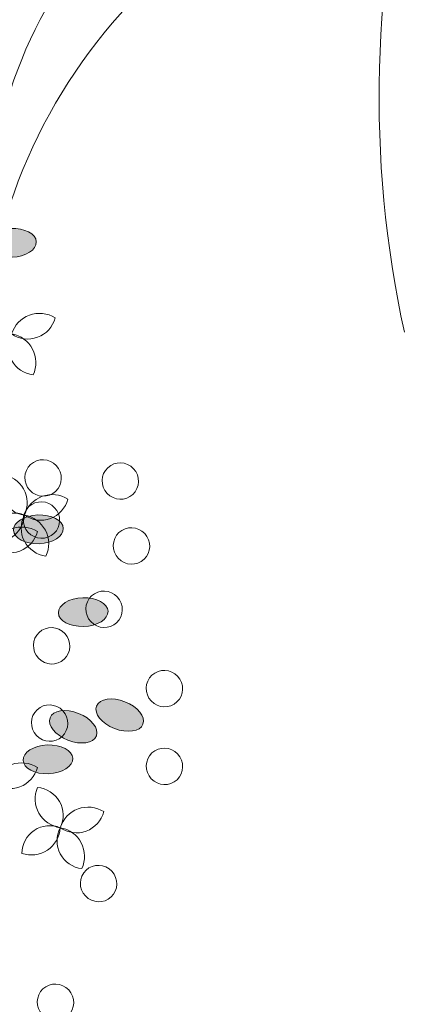
# Model space of a CAD drawing. Units: millimetres. Extents: x 595116 to 630915, y 909473 to 920225.
# Tile 47 of 134: x 629519 to 629529, y 919255 to 919281. Entities that reach past the tile are written whole.
import ezdxf

# ---------------------------------------------------------------- set-up
doc = ezdxf.new("R2010")
doc.units = ezdxf.units.MM
doc.layers.add('Dimension', color=3, linetype='Continuous', lineweight=18)
doc.layers.add('L-PLNT', color=85, linetype='Continuous', lineweight=13)
doc.styles.get("Standard").update_dxf_attribs({"font": 'arial.ttf'})
doc.dimstyles.new('ISO-25', dxfattribs={"dimtxt": 9, "dimasz": 6, "dimexe": 1.25, "dimexo": 0.625, "dimtad": 1, "dimlunit": 4, "dimtxsty": 'Standard', "dimcen": 2.5, "dimadec": 0, "dimazin": 0, "dimtfac": 1, "dimtmove": 0, "dimatfit": 3, "dimfxl": 1, "dimarcsym": 0})

# ---------------------------------------------------------------- blocks, each defined once
blk = doc.blocks.new('tree')
for centre, radius, start, end in [((629598.153, 919288.998), 5.103, 105.3576, 208.8973), ((629601.247, 919287.941), 5.545, 101.0419, 191.8692), ((629614.329, 919289.554), 13.748, 164.5925, 192.323), ((629602.391, 919286.088), 6.769, 99.681, 184.5451)]:
    blk.add_arc(centre, radius, start, end)
blk = doc.blocks.new('A$C77972600')
h = blk.add_hatch(color=256)
edge = h.paths.add_edge_path()
edge.add_ellipse((3.0705, 5.8276), major_axis=(-0.1731, 0.0699), ratio=0.578492, start_angle=0, end_angle=360)
edge = h.paths.add_edge_path()
edge.add_ellipse((4.0989, 6.0027), major_axis=(-0.1319, 0.1321), ratio=0.578492, start_angle=0, end_angle=360)
edge = h.paths.add_edge_path()
edge.add_ellipse((4.5318, 6.7683), major_axis=(-0.1688, -0.0798), ratio=0.578492, start_angle=0, end_angle=360)
edge = h.paths.add_edge_path()
edge.add_ellipse((5.185, 6.8705), major_axis=(-0.1865, -0.0073), ratio=0.578492, start_angle=0, end_angle=360)
edge = h.paths.add_edge_path()
edge.add_ellipse((4.6885, 3.4464), major_axis=(-0.1865, -0.0073), ratio=0.578492, start_angle=0, end_angle=360)
edge = h.paths.add_edge_path()
edge.add_ellipse((4.5217, 4.2367), major_axis=(-0.1865, -0.0073), ratio=0.578492, start_angle=0, end_angle=360)
edge = h.paths.add_edge_path()
edge.add_ellipse((4.9166, 3.9946), major_axis=(-0.1731, 0.0699), ratio=0.578492, start_angle=0, end_angle=360)
edge = h.paths.add_edge_path()
edge.add_ellipse((3.6759, 4.9988), major_axis=(-0.1319, 0.1321), ratio=0.578492, start_angle=0, end_angle=360)
edge = h.paths.add_edge_path()
edge.add_ellipse((3.1035, 4.6784), major_axis=(-0.1319, 0.1321), ratio=0.578492, start_angle=0, end_angle=360)
edge = h.paths.add_edge_path()
edge.add_ellipse((3.8133, 4.5577), major_axis=(-0.1319, 0.1321), ratio=0.578492, start_angle=0, end_angle=360)
edge = h.paths.add_edge_path()
edge.add_ellipse((2.2042, 5.6327), major_axis=(-0.1865, -0.0073), ratio=0.578492, start_angle=0, end_angle=360)
edge = h.paths.add_edge_path()
edge.add_ellipse((2.9066, 5.6543), major_axis=(-0.1865, -0.0073), ratio=0.578492, start_angle=0, end_angle=360)
edge = h.paths.add_edge_path()
edge.add_ellipse((2.6215, 5.4344), major_axis=(-0.1865, -0.0073), ratio=0.578492, start_angle=0, end_angle=360)
edge = h.paths.add_edge_path()
edge.add_ellipse((2.1195, 4.0174), major_axis=(-0.1731, 0.0699), ratio=0.578492, start_angle=0, end_angle=360)
edge = h.paths.add_edge_path()
edge.add_ellipse((4.1491, 5.5914), major_axis=(-0.1688, -0.0798), ratio=0.578492, start_angle=0, end_angle=360)
edge = h.paths.add_edge_path()
edge.add_ellipse((1.9571, 3.173), major_axis=(-0.1865, -0.0073), ratio=0.578492, start_angle=0, end_angle=360)
edge = h.paths.add_edge_path()
edge.add_ellipse((1.589, 3.2907), major_axis=(-0.1688, -0.0798), ratio=0.578492, start_angle=0, end_angle=360)
edge = h.paths.add_edge_path()
edge.add_ellipse((1.045, 3.0811), major_axis=(-0.1865, -0.0073), ratio=0.578492, start_angle=0, end_angle=360)
edge = h.paths.add_edge_path()
edge.add_ellipse((1.2104, 3.7739), major_axis=(-0.1688, -0.0798), ratio=0.578492, start_angle=0, end_angle=360)
edge = h.paths.add_edge_path()
edge.add_ellipse((1.6721, 3.755), major_axis=(-0.1688, -0.0798), ratio=0.578492, start_angle=0, end_angle=360)
edge = h.paths.add_edge_path()
edge.add_ellipse((0.772, 4.473), major_axis=(-0.1731, 0.0699), ratio=0.578492, start_angle=0, end_angle=360)
edge = h.paths.add_edge_path()
edge.add_ellipse((0.8326, 5.2916), major_axis=(-0.1319, 0.1321), ratio=0.578492, start_angle=0, end_angle=360)
edge = h.paths.add_edge_path()
edge.add_ellipse((1.1875, 5.2313), major_axis=(-0.1319, 0.1321), ratio=0.578492, start_angle=0, end_angle=360)
edge = h.paths.add_edge_path()
edge.add_ellipse((5.3876, 4.7197), major_axis=(-0.1865, -0.0073), ratio=0.578492, start_angle=0, end_angle=360)
edge = h.paths.add_edge_path()
edge.add_ellipse((3.5552, 2.162), major_axis=(-0.1865, -0.0073), ratio=0.578492, start_angle=0, end_angle=360)
edge = h.paths.add_edge_path()
edge.add_ellipse((3.8402, 2.3819), major_axis=(-0.1865, -0.0073), ratio=0.578492, start_angle=0, end_angle=360)
edge = h.paths.add_edge_path()
edge.add_ellipse((4.692, 2.204), major_axis=(-0.1731, 0.0699), ratio=0.578492, start_angle=0, end_angle=360)
edge = h.paths.add_edge_path()
edge.add_ellipse((4.514, 2.9096), major_axis=(-0.1731, 0.0699), ratio=0.578492, start_angle=0, end_angle=360)
edge = h.paths.add_edge_path()
edge.add_ellipse((4.8133, 2.5575), major_axis=(-0.1731, 0.0699), ratio=0.578492, start_angle=0, end_angle=360)
edge = h.paths.add_edge_path()
edge.add_ellipse((3.7876, 2.8899), major_axis=(-0.1731, 0.0699), ratio=0.578492, start_angle=0, end_angle=360)
h = blk.add_hatch(color=256)
edge = h.paths.add_edge_path()
edge.add_ellipse((3.2403, 1.6985), major_axis=(-0.1668, -0.0838), ratio=0.578492, start_angle=0, end_angle=360, ccw=False)
edge = h.paths.add_edge_path()
edge.add_ellipse((4.2796, 1.6084), major_axis=(-0.1206, -0.1425), ratio=0.578492, start_angle=0, end_angle=360, ccw=False)
edge = h.paths.add_edge_path()
edge.add_ellipse((4.7739, 0.881), major_axis=(-0.1747, 0.0657), ratio=0.578492, start_angle=0, end_angle=360, ccw=False)
edge = h.paths.add_edge_path()
edge.add_ellipse((5.4333, 0.8328), major_axis=(-0.1865, -0.008), ratio=0.578492, start_angle=0, end_angle=360, ccw=False)
edge = h.paths.add_edge_path()
edge.add_ellipse((4.6573, 4.2045), major_axis=(-0.1865, -0.008), ratio=0.578492, start_angle=0, end_angle=360, ccw=False)
edge = h.paths.add_edge_path()
edge.add_ellipse((4.556, 3.4032), major_axis=(-0.1865, -0.008), ratio=0.578492, start_angle=0, end_angle=360, ccw=False)
edge = h.paths.add_edge_path()
edge.add_ellipse((4.9297, 3.677), major_axis=(-0.1668, -0.0838), ratio=0.578492, start_angle=0, end_angle=360, ccw=False)
edge = h.paths.add_edge_path()
edge.add_ellipse((3.7756, 2.5742), major_axis=(-0.1206, -0.1425), ratio=0.578492, start_angle=0, end_angle=360, ccw=False)
edge = h.paths.add_edge_path()
edge.add_ellipse((3.1788, 2.8466), major_axis=(-0.1206, -0.1425), ratio=0.578492, start_angle=0, end_angle=360, ccw=False)
edge = h.paths.add_edge_path()
edge.add_ellipse((3.8763, 3.0252), major_axis=(-0.1206, -0.1425), ratio=0.578492, start_angle=0, end_angle=360, ccw=False)
edge = h.paths.add_edge_path()
edge.add_ellipse((2.3609, 1.8217), major_axis=(-0.1865, -0.008), ratio=0.578492, start_angle=0, end_angle=360, ccw=False)
edge = h.paths.add_edge_path()
edge.add_ellipse((3.0627, 1.8578), major_axis=(-0.1865, -0.008), ratio=0.578492, start_angle=0, end_angle=360, ccw=False)
edge = h.paths.add_edge_path()
edge.add_ellipse((2.7605, 2.0535), major_axis=(-0.1865, -0.008), ratio=0.578492, start_angle=0, end_angle=360, ccw=False)
edge = h.paths.add_edge_path()
edge.add_ellipse((2.1439, 3.4246), major_axis=(-0.1668, -0.0838), ratio=0.578492, start_angle=0, end_angle=360, ccw=False)
edge = h.paths.add_edge_path()
edge.add_ellipse((4.2959, 2.0225), major_axis=(-0.1747, 0.0657), ratio=0.578492, start_angle=0, end_angle=360, ccw=False)
edge = h.paths.add_edge_path()
edge.add_ellipse((1.9127, 4.2528), major_axis=(-0.1865, -0.008), ratio=0.578492, start_angle=0, end_angle=360, ccw=False)
edge = h.paths.add_edge_path()
edge.add_ellipse((1.5555, 4.1052), major_axis=(-0.1747, 0.0657), ratio=0.578492, start_angle=0, end_angle=360, ccw=False)
edge = h.paths.add_edge_path()
edge.add_ellipse((0.9962, 4.2695), major_axis=(-0.1865, -0.008), ratio=0.578492, start_angle=0, end_angle=360, ccw=False)
edge = h.paths.add_edge_path()
edge.add_ellipse((1.2179, 3.5926), major_axis=(-0.1747, 0.0657), ratio=0.578492, start_angle=0, end_angle=360, ccw=False)
edge = h.paths.add_edge_path()
edge.add_ellipse((1.6764, 3.6493), major_axis=(-0.1747, 0.0657), ratio=0.578492, start_angle=0, end_angle=360, ccw=False)
edge = h.paths.add_edge_path()
edge.add_ellipse((0.8384, 2.8599), major_axis=(-0.1668, -0.0838), ratio=0.578492, start_angle=0, end_angle=360, ccw=False)
edge = h.paths.add_edge_path()
edge.add_ellipse((0.9659, 2.049), major_axis=(-0.1206, -0.1425), ratio=0.578492, start_angle=0, end_angle=360, ccw=False)
edge = h.paths.add_edge_path()
edge.add_ellipse((1.3147, 2.1383), major_axis=(-0.1206, -0.1425), ratio=0.578492, start_angle=0, end_angle=360, ccw=False)
edge = h.paths.add_edge_path()
edge.add_ellipse((5.4586, 2.9929), major_axis=(-0.1865, -0.008), ratio=0.578492, start_angle=0, end_angle=360, ccw=False)
edge = h.paths.add_edge_path()
edge.add_ellipse((3.4224, 5.3915), major_axis=(-0.1865, -0.008), ratio=0.578492, start_angle=0, end_angle=360, ccw=False)
edge = h.paths.add_edge_path()
edge.add_ellipse((3.7245, 5.1958), major_axis=(-0.1865, -0.008), ratio=0.578492, start_angle=0, end_angle=360, ccw=False)
edge = h.paths.add_edge_path()
edge.add_ellipse((4.5588, 5.4431), major_axis=(-0.1668, -0.0838), ratio=0.578492, start_angle=0, end_angle=360, ccw=False)
edge = h.paths.add_edge_path()
edge.add_ellipse((4.4393, 4.7252), major_axis=(-0.1668, -0.0838), ratio=0.578492, start_angle=0, end_angle=360, ccw=False)
edge = h.paths.add_edge_path()
edge.add_ellipse((4.7087, 5.1006), major_axis=(-0.1668, -0.0838), ratio=0.578492, start_angle=0, end_angle=360, ccw=False)
edge = h.paths.add_edge_path()
edge.add_ellipse((3.7138, 4.6852), major_axis=(-0.1668, -0.0838), ratio=0.578492, start_angle=0, end_angle=360, ccw=False)
h = blk.add_hatch(color=256)
edge = h.paths.add_edge_path()
edge.add_ellipse((4.1652, 1.933), major_axis=(0.1866, 0.0058), ratio=0.578492, start_angle=0, end_angle=360)
edge = h.paths.add_edge_path()
edge.add_ellipse((3.2944, 1.3586), major_axis=(0.1739, -0.0678), ratio=0.578492, start_angle=0, end_angle=360)
edge = h.paths.add_edge_path()
edge.add_ellipse((3.2064, 0.4835), major_axis=(0.1223, 0.141), ratio=0.578492, start_angle=0, end_angle=360)
edge = h.paths.add_edge_path()
edge.add_ellipse((2.6497, 0.127), major_axis=(0.1678, 0.0818), ratio=0.578492, start_angle=0, end_angle=360)
edge = h.paths.add_edge_path()
edge.add_ellipse((1.7252, 3.461), major_axis=(0.1678, 0.0818), ratio=0.578492, start_angle=0, end_angle=360)
edge = h.paths.add_edge_path()
edge.add_ellipse((2.1962, 2.8048), major_axis=(0.1678, 0.0818), ratio=0.578492, start_angle=0, end_angle=360)
edge = h.paths.add_edge_path()
edge.add_ellipse((1.7372, 2.8674), major_axis=(0.1866, 0.0058), ratio=0.578492, start_angle=0, end_angle=360)
edge = h.paths.add_edge_path()
edge.add_ellipse((3.2773, 2.4479), major_axis=(0.1739, -0.0678), ratio=0.578492, start_angle=0, end_angle=360)
edge = h.paths.add_edge_path()
edge.add_ellipse((3.6722, 2.9717), major_axis=(0.1739, -0.0678), ratio=0.578492, start_angle=0, end_angle=360)
edge = h.paths.add_edge_path()
edge.add_ellipse((2.9739, 2.7963), major_axis=(0.1739, -0.0678), ratio=0.578492, start_angle=0, end_angle=360)
edge = h.paths.add_edge_path()
edge.add_ellipse((4.8796, 2.4604), major_axis=(0.1678, 0.0818), ratio=0.578492, start_angle=0, end_angle=360)
edge = h.paths.add_edge_path()
edge.add_ellipse((4.2454, 2.1577), major_axis=(0.1678, 0.0818), ratio=0.578492, start_angle=0, end_angle=360)
edge = h.paths.add_edge_path()
edge.add_ellipse((4.4178, 2.4738), major_axis=(0.1678, 0.0818), ratio=0.578492, start_angle=0, end_angle=360)
edge = h.paths.add_edge_path()
edge.add_ellipse((4.3066, 3.973), major_axis=(0.1866, 0.0058), ratio=0.578492, start_angle=0, end_angle=360)
edge = h.paths.add_edge_path()
edge.add_ellipse((3.0828, 1.7149), major_axis=(0.1223, 0.141), ratio=0.578492, start_angle=0, end_angle=360)
edge = h.paths.add_edge_path()
edge.add_ellipse((4.1152, 4.8113), major_axis=(0.1678, 0.0818), ratio=0.578492, start_angle=0, end_angle=360)
edge = h.paths.add_edge_path()
edge.add_ellipse((4.4995, 4.8518), major_axis=(0.1223, 0.141), ratio=0.578492, start_angle=0, end_angle=360)
edge = h.paths.add_edge_path()
edge.add_ellipse((4.913, 5.2627), major_axis=(0.1678, 0.0818), ratio=0.578492, start_angle=0, end_angle=360)
edge = h.paths.add_edge_path()
edge.add_ellipse((5.0407, 4.562), major_axis=(0.1223, 0.141), ratio=0.578492, start_angle=0, end_angle=360)
edge = h.paths.add_edge_path()
edge.add_ellipse((4.6105, 4.3933), major_axis=(0.1223, 0.141), ratio=0.578492, start_angle=0, end_angle=360)
edge = h.paths.add_edge_path()
edge.add_ellipse((5.7235, 4.0986), major_axis=(0.1866, 0.0058), ratio=0.578492, start_angle=0, end_angle=360)
edge = h.paths.add_edge_path()
edge.add_ellipse((5.9977, 3.3249), major_axis=(0.1739, -0.0678), ratio=0.578492, start_angle=0, end_angle=360)
edge = h.paths.add_edge_path()
edge.add_ellipse((5.6486, 3.2372), major_axis=(0.1739, -0.0678), ratio=0.578492, start_angle=0, end_angle=360)
edge = h.paths.add_edge_path()
edge.add_ellipse((1.5981, 2.014), major_axis=(0.1678, 0.0818), ratio=0.578492, start_angle=0, end_angle=360)
edge = h.paths.add_edge_path()
edge.add_ellipse((2.2453, 5.0931), major_axis=(0.1678, 0.0818), ratio=0.578492, start_angle=0, end_angle=360)
edge = h.paths.add_edge_path()
edge.add_ellipse((2.073, 4.777), major_axis=(0.1678, 0.0818), ratio=0.578492, start_angle=0, end_angle=360)
edge = h.paths.add_edge_path()
edge.add_ellipse((1.2216, 4.5968), major_axis=(0.1866, 0.0058), ratio=0.578492, start_angle=0, end_angle=360)
edge = h.paths.add_edge_path()
edge.add_ellipse((1.6688, 4.0227), major_axis=(0.1866, 0.0058), ratio=0.578492, start_angle=0, end_angle=360)
edge = h.paths.add_edge_path()
edge.add_ellipse((1.253, 4.2244), major_axis=(0.1866, 0.0058), ratio=0.578492, start_angle=0, end_angle=360)
edge = h.paths.add_edge_path()
edge.add_ellipse((2.3257, 4.3332), major_axis=(0.1866, 0.0058), ratio=0.578492, start_angle=0, end_angle=360)
for centre, radius, start, end in [((5.3953, 6.1226), 0.2185, 57.5868, 162.92381), ((5.3082, 6.3586), 0.2106, 234.66708, 345.84353), ((5.3726, 6.0884), 0.2106, 152.13841, 263.31486), ((5.1499, 5.9713), 0.2185, 335.05813, 80.39514), ((5.3122, 5.0432), 0.2185, 156.8071, 262.14411), ((5.0932, 4.9194), 0.2106, 333.88738, 85.06383), ((5.4913, 4.7625), 0.2185, 57.5868, 162.92381), ((5.4042, 4.9985), 0.2106, 234.66708, 345.84353), ((5.204, 4.6312), 0.2106, 68.14697, 179.32342), ((5.0643, 4.8404), 0.2185, 251.0667, 356.4037), ((5.4686, 4.7282), 0.2106, 152.13841, 263.31486), ((5.2459, 4.6112), 0.2185, 335.05813, 80.39514), ((5.2625, 4.5183), 0.2185, 57.5868, 162.92381), ((5.1754, 4.7544), 0.2106, 234.66708, 345.84353), ((5.2625, 2.7483), 0.2185, 57.5868, 162.92381), ((5.1754, 2.9843), 0.2106, 234.66708, 345.84353), ((5.5815, 2.6965), 0.2185, 156.8071, 262.14411), ((5.3625, 2.5727), 0.2106, 333.88738, 85.06383), ((5.7605, 2.4158), 0.2185, 57.5868, 162.92381), ((5.6734, 2.6518), 0.2106, 234.66708, 345.84353), ((5.4732, 2.2845), 0.2106, 68.14697, 179.32342), ((5.3335, 2.4937), 0.2185, 251.0667, 356.4037), ((5.7378, 2.3816), 0.2106, 152.13841, 263.31486), ((5.5151, 2.2645), 0.2185, 335.05813, 80.39514)]:
    blk.add_arc(centre, radius, start, end)
for centre, major_axis, start_param, end_param in [((5.185, 6.8705), (-0.1865, -0.0073), 1.570796326839852, 7.853981634019438), ((5.3876, 4.7197), (-0.1865, -0.0073), 1.570796326819928, 7.853981633999514), ((5.7235, 4.0986), (-0.1866, -0.0058), 4.712389, 10.995574), ((5.9977, 3.3249), (-0.1739, 0.0678), 3.141593, 9.424778), ((5.6486, 3.2372), (-0.1739, 0.0678), 3.141593, 9.424778)]:
    blk.add_ellipse(centre, major_axis=major_axis, ratio=0.578492, start_param=start_param, end_param=end_param)
for centre in [(5.4223, 5.1054), (6.0019, 5.0821), (5.4098, 4.7894), (6.086, 4.595), (5.8803, 4.1195), (5.4865, 3.8451), (6.3331, 3.524), (5.4715, 3.2652), (6.3334, 2.9404), (5.8392, 2.0603), (5.5155, 1.1693)]:
    blk.add_ellipse(centre, major_axis=(-0.0941, 0.1005), ratio=0.985729)
at = {"extrusion": (0, 0, -1)}
blk.add_ellipse((5.4586, 2.9929), major_axis=(-0.1865, -0.008), ratio=0.578492, start_param=3.141593, end_param=9.424778, dxfattribs=at)
blk = doc.blocks.new('*D216')
at = {"layer": 'Defpoints', "color": 0, "transparency": 16777216}
for p in [(629743.541, 919411.928), (629505.041, 919411.828), (629743.541, 918832.378)]:
    blk.add_point(p, dxfattribs=at)
at = {"layer": 'Dimension', "color": 0, "lineweight": -2, "transparency": 16777216}
for p, q in [((629505.041, 919411.203), (629505.041, 918831.128)), ((629743.541, 919411.303), (629743.541, 918831.128)), ((629511.041, 918832.378), (629737.541, 918832.378))]:
    blk.add_line(p, q, dxfattribs=at)
at = {"layer": 'Dimension', "color": 0, "transparency": 16777216}
for points in [[(629511.041, 918833.378), (629511.041, 918831.378), (629505.041, 918832.378)], [(629737.541, 918833.378), (629737.541, 918831.378), (629743.541, 918832.378)]]:
    blk.add_solid(points, dxfattribs=at)
at = {"layer": 'Dimension', "color": 0, "transparency": 16777216, "insert": (629624.291, 918837.656), "char_height": 9, "attachment_point": 5}
blk.add_mtext('19\'-10 1/2"', dxfattribs=at)

msp = doc.modelspace()

# ---------------------------------------------------------------- block references
at = {"layer": 'L-PLNT'}
for name, p, xscale, yscale, zscale in [('tree', (-697473.9, -1018297.752), 2.107689410566463, 2.107689410566463, 2.107689410566463), ('A$C77972600', (629500.673, 919251.142), 3.512546757812034, 3.512546757812034, 3.512546757812034)]:
    msp.add_blockref(name, p, dxfattribs=dict(at, xscale=xscale, yscale=yscale, zscale=zscale))

# ---------------------------------------------------------------- dimensions: what is measured, and where the dimension line sits
at = {"layer": 'Dimension'}
dim = msp.add_linear_dim(base=(629743.541, 918832.378), p1=(629505.041, 919411.828), p2=(629743.541, 919411.928), dimstyle='ISO-25', override={"dimdec": 1, "dimlfac": 1, "dimrnd": 0, "dimzin": 1, "dimdsep": 46, "dimlunit": 4, "dimfrac": 2}, dxfattribs=at)
dim.commit()
dim.dimension.update_dxf_attribs({"geometry": '*D216', "text_midpoint": (629624.291, 918837.656)})

doc.saveas('drawing.dxf')
